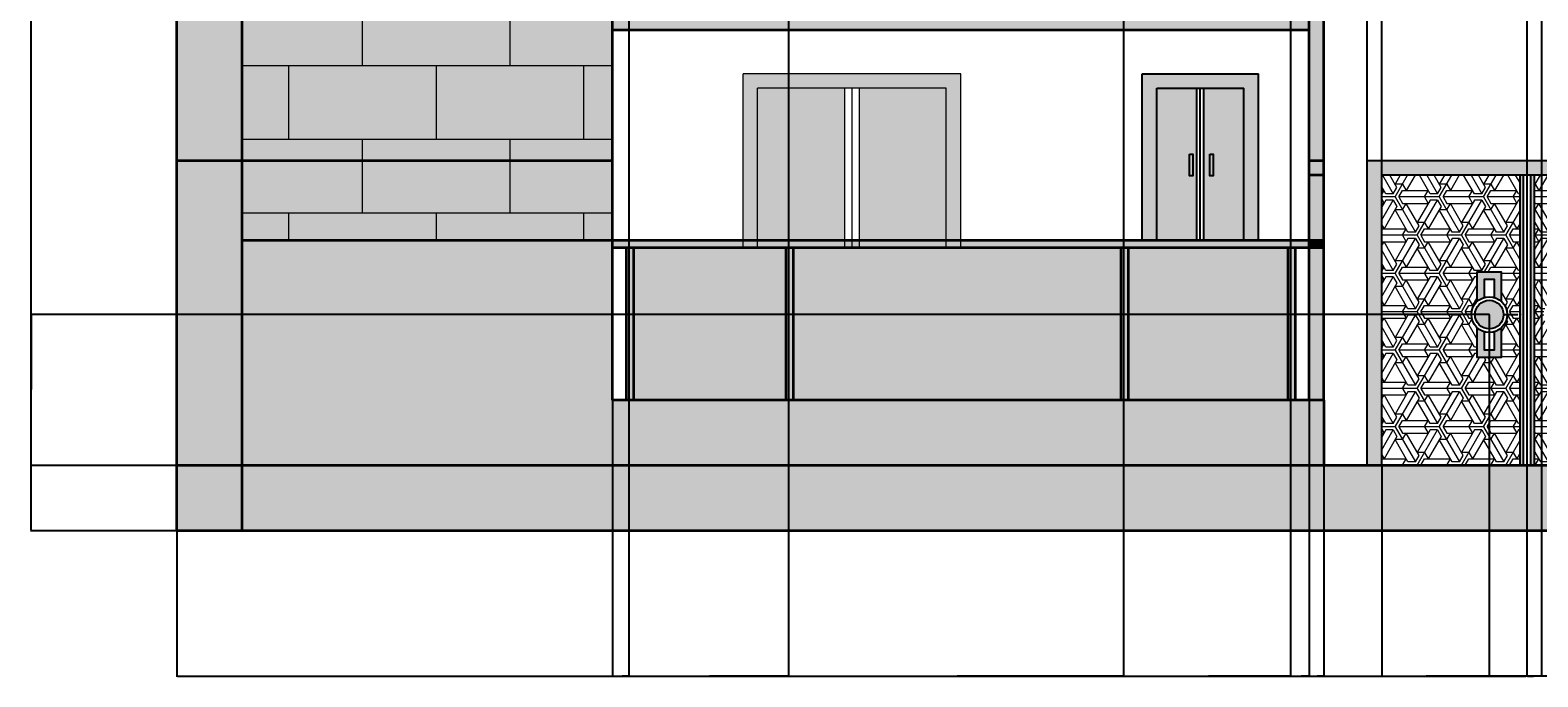
# Model space of a CAD drawing. Units: inches. Extents: x 2794 to 3619, y 522 to 1397.
# Tile 1 of 10: x 2794 to 3209, y 522 to 701. Entities that reach past the tile are written whole.
import ezdxf

# ---------------------------------------------------------------- set-up
doc = ezdxf.new("R2010")
doc.units = ezdxf.units.IN
for name, color, linetype, lineweight in [('A-ANNO-DIMS', 2, 'Continuous', 18), ('A-DOOR', 3, 'Continuous', 25), ('A-ELEV', 7, 'Continuous', 35), ('A-ELEV-PATT', 8, 'Continuous', 13), ('A-GLAZ', 4, 'Continuous', 18)]:
    doc.layers.add(name, color=color, linetype=linetype, lineweight=lineweight)
doc.styles.get("Standard").update_dxf_attribs({"font": 'arial.ttf'})
doc.dimstyles.get("Standard").update_dxf_attribs({"dimtxt": 0.18, "dimasz": 0.18, "dimexe": 0.18, "dimexo": 0.0625, "dimgap": 0.09, "dimtad": 0, "dimtih": 1, "dimtoh": 1, "dimdec": 4, "dimzin": 0, "dimdsep": 46, "dimtxsty": 'Standard', "dimcen": 0.09, "dimadec": 0, "dimazin": 0, "dimtfac": 1, "dimtdec": 4, "dimtofl": 0, "dimtmove": 0, "dimatfit": 3, "dimfxl": 1, "dimtolj": 1, "dimtzin": 0, "dimarcsym": 0})

# ---------------------------------------------------------------- blocks, each defined once
blk = doc.blocks.new('WIN-1500')
at = {"transparency": 33554646}
h = blk.add_hatch(color=256, dxfattribs=at)
h.dxf.hatch_style = 1
h.paths.add_polyline_path([(60, 48), (0, 48), (0, 2), (4, 2), (4, 44), (56, 44), (56, 2), (60, 2)])
at = {"transparency": 33554687}
h = blk.add_hatch(color=256, dxfattribs=at)
h.dxf.hatch_style = 1
h.set_gradient(color1=(248, 246, 176), color2=(74, 13, 14), name='INVCYLINDER')
h.paths.add_polyline_path([(56, 44), (32, 44), (32, 2), (56, 2)])
h.paths.add_polyline_path([(28, 44), (4, 44), (4, 2), (28, 2)])
for p, q in [((0, 0), (0, 48)), ((60, 48), (0, 48)), ((60, 0), (60, 48)), ((56, 44), (4, 44)), ((4, 0), (4, 44)), ((28, 44), (28, 0)), ((30, 44), (30, 0)), ((32, 44), (32, 0)), ((56, 0), (56, 44))]:
    blk.add_line(p, q)
blk = doc.blocks.new('DOOR-BALCONY-DBL')
at = {"transparency": 33554628}
h = blk.add_hatch(color=256, dxfattribs=at)
h.dxf.hatch_style = 1
h.paths.add_polyline_path([(4, 42), (28, 42), (28, 0), (32, 0), (32, 46), (0, 46), (0, 0), (4, 0)])
at = {"transparency": 33554646}
h = blk.add_hatch(color=256, dxfattribs=at)
h.dxf.hatch_style = 1
h.set_gradient(color1=(255, 255, 255), color2=(147, 149, 152), name='INVCYLINDER')
h.paths.add_polyline_path([(15, 42), (4, 42), (4, 0), (15, 0)])
h = blk.add_hatch(color=256, dxfattribs=at)
h.dxf.hatch_style = 1
h.set_gradient(color1=(255, 255, 255), color2=(147, 149, 152), name='INVCYLINDER')
h.paths.add_polyline_path([(28, 42), (17, 42), (17, 0), (28, 0)])
for p, q in [((0, 0), (0, 46)), ((0, 46), (32, 46)), ((4, 46), (28, 46)), ((32, 0), (32, 46)), ((4, 0), (4, 42)), ((4, 42), (28, 42)), ((15, 0), (15, 42)), ((16, 0), (16, 42)), ((17, 0), (17, 42)), ((28, 0), (28, 42))]:
    blk.add_line(p, q)
for points in [[(12.99, 23.83), (13.93, 23.83), (13.93, 17.87), (12.99, 17.87)], [(18.59, 23.83), (19.53, 23.83), (19.53, 17.87), (18.59, 17.87)]]:
    blk.add_lwpolyline(points, close=True)
blk = doc.blocks.new('*D7')
at = {"layer": 'A-ANNO-DIMS', "color": 0, "lineweight": -2, "transparency": 16777216}
for p, q in [((2834.27, 562.57), (2834.27, 522.36)), ((3578.27, 562.57), (3578.27, 522.36)), ((2834.45, 522.54), (3205.98, 522.54)), ((3578.09, 522.54), (3206.55, 522.54))]:
    blk.add_line(p, q, dxfattribs=at)
at = {"layer": 'A-ANNO-DIMS', "color": 0, "transparency": 16777216}
for points in [[(2834.45, 522.57), (2834.45, 522.51), (2834.27, 522.54)], [(3578.09, 522.57), (3578.09, 522.51), (3578.27, 522.54)]]:
    blk.add_solid(points, dxfattribs=at)
at = {"layer": 'Defpoints', "color": 0, "transparency": 16777216}
for p in [(2834.27, 562.64), (3578.27, 562.64), (3578.27, 522.54)]:
    blk.add_point(p, dxfattribs=at)
at = {"layer": 'A-ANNO-DIMS', "color": 0, "transparency": 16777216, "insert": (3206.27, 522.54), "char_height": 0.18, "attachment_point": 5}
blk.add_mtext('\\A1;744', dxfattribs=at)
blk = doc.blocks.new('*D16')
at = {"layer": 'A-ANNO-DIMS', "color": 0, "lineweight": -2, "transparency": 16777216}
for p, q in [((3142.2, 1356.64), (2793.99, 1356.64)), ((2794.17, 1356.46), (2794.17, 959.82)), ((2794.17, 562.82), (2794.17, 959.45)), ((2834.2, 562.64), (2793.99, 562.64))]:
    blk.add_line(p, q, dxfattribs=at)
at = {"layer": 'A-ANNO-DIMS', "color": 0, "transparency": 16777216}
for points in [[(2794.14, 1356.46), (2794.2, 1356.46), (2794.17, 1356.64)], [(2794.14, 562.82), (2794.2, 562.82), (2794.17, 562.64)]]:
    blk.add_solid(points, dxfattribs=at)
at = {"layer": 'Defpoints', "color": 0, "transparency": 16777216}
for p in [(2794.17, 1356.64), (3142.27, 1356.64), (2834.27, 562.64)]:
    blk.add_point(p, dxfattribs=at)
at = {"layer": 'A-ANNO-DIMS', "color": 0, "transparency": 16777216, "insert": (2794.17, 959.64), "char_height": 0.18, "attachment_point": 5}
blk.add_mtext('\\A1;794', dxfattribs=at)
blk = doc.blocks.new('*D32')
at = {"layer": 'A-ANNO-DIMS', "color": 0, "lineweight": -2, "transparency": 16777216}
for p, q in [((2954.27, 772.57), (2954.27, 522.36)), ((2958.83, 730.57), (2958.83, 522.36)), ((2954.45, 522.54), (2956.17, 522.54)), ((2958.65, 522.54), (2956.93, 522.54))]:
    blk.add_line(p, q, dxfattribs=at)
at = {"layer": 'A-ANNO-DIMS', "color": 0, "transparency": 16777216}
for points in [[(2954.45, 522.57), (2954.45, 522.51), (2954.27, 522.54)], [(2958.65, 522.57), (2958.65, 522.51), (2958.83, 522.54)]]:
    blk.add_solid(points, dxfattribs=at)
at = {"layer": 'Defpoints', "color": 0, "transparency": 16777216}
for p in [(2954.27, 772.64), (2958.83, 730.64), (2958.83, 522.54)]:
    blk.add_point(p, dxfattribs=at)
at = {"layer": 'A-ANNO-DIMS', "color": 0, "transparency": 16777216, "insert": (2956.55, 522.54), "char_height": 0.18, "attachment_point": 5}
blk.add_mtext('\\A1;4.561', dxfattribs=at)
blk = doc.blocks.new('*D33')
at = {"layer": 'A-ANNO-DIMS', "color": 0, "lineweight": -2, "transparency": 16777216}
for p, q in [((2958.83, 730.57), (2958.83, 522.36)), ((3002.83, 730.57), (3002.83, 522.36)), ((2959.01, 522.54), (2980.6, 522.54)), ((3002.65, 522.54), (2981.05, 522.54))]:
    blk.add_line(p, q, dxfattribs=at)
at = {"layer": 'A-ANNO-DIMS', "color": 0, "transparency": 16777216}
for points in [[(2959.01, 522.57), (2959.01, 522.51), (2958.83, 522.54)], [(3002.65, 522.57), (3002.65, 522.51), (3002.83, 522.54)]]:
    blk.add_solid(points, dxfattribs=at)
at = {"layer": 'Defpoints', "color": 0, "transparency": 16777216}
for p in [(2958.83, 730.64), (3002.83, 730.64), (3002.83, 522.54)]:
    blk.add_point(p, dxfattribs=at)
at = {"layer": 'A-ANNO-DIMS', "color": 0, "transparency": 16777216, "insert": (2980.83, 522.54), "char_height": 0.18, "attachment_point": 5}
blk.add_mtext('\\A1;44', dxfattribs=at)
blk = doc.blocks.new('*D34')
at = {"layer": 'A-ANNO-DIMS', "color": 0, "lineweight": -2, "transparency": 16777216}
for p, q in [((3002.83, 730.57), (3002.83, 522.36)), ((3095.13, 730.57), (3095.13, 522.36)), ((3003.01, 522.54), (3048.66, 522.54)), ((3094.95, 522.54), (3049.3, 522.54))]:
    blk.add_line(p, q, dxfattribs=at)
at = {"layer": 'A-ANNO-DIMS', "color": 0, "transparency": 16777216}
for points in [[(3003.01, 522.57), (3003.01, 522.51), (3002.83, 522.54)], [(3094.95, 522.57), (3094.95, 522.51), (3095.13, 522.54)]]:
    blk.add_solid(points, dxfattribs=at)
at = {"layer": 'Defpoints', "color": 0, "transparency": 16777216}
for p in [(3002.83, 730.64), (3095.13, 730.64), (3095.13, 522.54)]:
    blk.add_point(p, dxfattribs=at)
at = {"layer": 'A-ANNO-DIMS', "color": 0, "transparency": 16777216, "insert": (3048.98, 522.54), "char_height": 0.18, "attachment_point": 5}
blk.add_mtext('\\A1;92.3', dxfattribs=at)
blk = doc.blocks.new('*D35')
at = {"layer": 'A-ANNO-DIMS', "color": 0, "lineweight": -2, "transparency": 16777216}
for p, q in [((3095.13, 730.57), (3095.13, 522.36)), ((3141.11, 730.57), (3141.11, 522.36)), ((3095.31, 522.54), (3117.72, 522.54)), ((3140.93, 522.54), (3118.52, 522.54))]:
    blk.add_line(p, q, dxfattribs=at)
at = {"layer": 'A-ANNO-DIMS', "color": 0, "transparency": 16777216}
for points in [[(3095.31, 522.57), (3095.31, 522.51), (3095.13, 522.54)], [(3140.93, 522.57), (3140.93, 522.51), (3141.11, 522.54)]]:
    blk.add_solid(points, dxfattribs=at)
at = {"layer": 'Defpoints', "color": 0, "transparency": 16777216}
for p in [(3095.13, 730.64), (3141.11, 730.64), (3141.11, 522.54)]:
    blk.add_point(p, dxfattribs=at)
at = {"layer": 'A-ANNO-DIMS', "color": 0, "transparency": 16777216, "insert": (3118.12, 522.54), "char_height": 0.18, "attachment_point": 5}
blk.add_mtext('\\A1;45.98', dxfattribs=at)
blk = doc.blocks.new('*D36')
at = {"layer": 'A-ANNO-DIMS', "color": 0, "lineweight": -2, "transparency": 16777216}
for p, q in [((3146.27, 772.57), (3146.27, 522.36)), ((3141.11, 730.57), (3141.11, 522.36)), ((3141.29, 522.54), (3143.3, 522.54)), ((3146.09, 522.54), (3144.08, 522.54))]:
    blk.add_line(p, q, dxfattribs=at)
at = {"layer": 'A-ANNO-DIMS', "color": 0, "transparency": 16777216}
for points in [[(3141.29, 522.57), (3141.29, 522.51), (3141.11, 522.54)], [(3146.09, 522.57), (3146.09, 522.51), (3146.27, 522.54)]]:
    blk.add_solid(points, dxfattribs=at)
at = {"layer": 'Defpoints', "color": 0, "transparency": 16777216}
for p in [(3146.27, 772.64), (3141.11, 730.64), (3146.27, 522.54)]:
    blk.add_point(p, dxfattribs=at)
at = {"layer": 'A-ANNO-DIMS', "color": 0, "transparency": 16777216, "insert": (3143.69, 522.54), "char_height": 0.18, "attachment_point": 5}
blk.add_mtext('\\A1;5.154', dxfattribs=at)
blk = doc.blocks.new('*D49')
at = {"layer": 'A-ANNO-DIMS', "color": 0, "lineweight": -2, "transparency": 16777216}
for p, q in [((3146.27, 1256.19), (3146.27, 522.36)), ((3150.27, 1254.57), (3150.27, 522.36)), ((3146.45, 522.54), (3148.11, 522.54)), ((3150.09, 522.54), (3148.42, 522.54))]:
    blk.add_line(p, q, dxfattribs=at)
at = {"layer": 'A-ANNO-DIMS', "color": 0, "transparency": 16777216}
for points in [[(3146.45, 522.57), (3146.45, 522.51), (3146.27, 522.54)], [(3150.09, 522.57), (3150.09, 522.51), (3150.27, 522.54)]]:
    blk.add_solid(points, dxfattribs=at)
at = {"layer": 'Defpoints', "color": 0, "transparency": 16777216}
for p in [(3146.27, 1256.25), (3150.27, 1254.64), (3150.27, 522.54)]:
    blk.add_point(p, dxfattribs=at)
at = {"layer": 'A-ANNO-DIMS', "color": 0, "transparency": 16777216, "insert": (3148.27, 522.54), "char_height": 0.18, "attachment_point": 5}
blk.add_mtext('\\A1;4', dxfattribs=at)
blk = doc.blocks.new('*D50')
at = {"layer": 'A-ANNO-DIMS', "color": 0, "lineweight": -2, "transparency": 16777216}
for p, q in [((3150.27, 1254.57), (3150.27, 522.36)), ((3206.27, 1254.57), (3206.27, 522.36)), ((3150.45, 522.54), (3178.05, 522.54)), ((3206.09, 522.54), (3178.48, 522.54))]:
    blk.add_line(p, q, dxfattribs=at)
at = {"layer": 'A-ANNO-DIMS', "color": 0, "transparency": 16777216}
for points in [[(3150.45, 522.57), (3150.45, 522.51), (3150.27, 522.54)], [(3206.09, 522.57), (3206.09, 522.51), (3206.27, 522.54)]]:
    blk.add_solid(points, dxfattribs=at)
at = {"layer": 'Defpoints', "color": 0, "transparency": 16777216}
for p in [(3150.27, 1254.64), (3206.27, 1254.64), (3206.27, 522.54)]:
    blk.add_point(p, dxfattribs=at)
at = {"layer": 'A-ANNO-DIMS', "color": 0, "transparency": 16777216, "insert": (3178.27, 522.54), "char_height": 0.18, "attachment_point": 5}
blk.add_mtext('\\A1;56', dxfattribs=at)
blk = doc.blocks.new('*D51')
at = {"layer": 'A-ANNO-DIMS', "color": 0, "lineweight": -2, "transparency": 16777216}
for p, q in [((3206.27, 1254.57), (3206.27, 522.36)), ((3210.27, 1254.57), (3210.27, 522.36)), ((3206.45, 522.54), (3208.11, 522.54)), ((3210.09, 522.54), (3208.42, 522.54))]:
    blk.add_line(p, q, dxfattribs=at)
at = {"layer": 'A-ANNO-DIMS', "color": 0, "transparency": 16777216}
for points in [[(3206.45, 522.57), (3206.45, 522.51), (3206.27, 522.54)], [(3210.09, 522.57), (3210.09, 522.51), (3210.27, 522.54)]]:
    blk.add_solid(points, dxfattribs=at)
at = {"layer": 'Defpoints', "color": 0, "transparency": 16777216}
for p in [(3206.27, 1254.64), (3210.27, 1254.64), (3210.27, 522.54)]:
    blk.add_point(p, dxfattribs=at)
at = {"layer": 'A-ANNO-DIMS', "color": 0, "transparency": 16777216, "insert": (3208.27, 522.54), "char_height": 0.18, "attachment_point": 5}
blk.add_mtext('\\A1;4', dxfattribs=at)
blk = doc.blocks.new('*D56')
at = {"layer": 'A-ANNO-DIMS', "color": 0, "lineweight": -2, "transparency": 16777216}
for p, q in [((3162.27, 664.7), (3162.27, 1396.92)), ((3162.45, 1396.74), (3206.05, 1396.74)), ((3250.09, 1396.74), (3206.49, 1396.74)), ((3250.27, 664.7), (3250.27, 1396.92))]:
    blk.add_line(p, q, dxfattribs=at)
at = {"layer": 'A-ANNO-DIMS', "color": 0, "transparency": 16777216}
for points in [[(3162.45, 1396.77), (3162.45, 1396.71), (3162.27, 1396.74)], [(3250.09, 1396.77), (3250.09, 1396.71), (3250.27, 1396.74)]]:
    blk.add_solid(points, dxfattribs=at)
at = {"layer": 'Defpoints', "color": 0, "transparency": 16777216}
for p in [(3250.27, 1396.74), (3162.27, 664.64), (3250.27, 664.64)]:
    blk.add_point(p, dxfattribs=at)
at = {"layer": 'A-ANNO-DIMS', "color": 0, "transparency": 16777216, "insert": (3206.27, 1396.74), "char_height": 0.18, "attachment_point": 5}
blk.add_mtext('\\A1;88', dxfattribs=at)
blk = doc.blocks.new('*D57')
at = {"layer": 'A-ANNO-DIMS', "color": 0, "lineweight": -2, "transparency": 16777216}
for p, q in [((3162.27, 664.7), (3162.27, 1396.92)), ((3162.45, 1396.74), (3164.11, 1396.74)), ((3166.09, 1396.74), (3164.42, 1396.74)), ((3166.27, 660.7), (3166.27, 1396.92))]:
    blk.add_line(p, q, dxfattribs=at)
at = {"layer": 'A-ANNO-DIMS', "color": 0, "transparency": 16777216}
for points in [[(3162.45, 1396.77), (3162.45, 1396.71), (3162.27, 1396.74)], [(3166.09, 1396.77), (3166.09, 1396.71), (3166.27, 1396.74)]]:
    blk.add_solid(points, dxfattribs=at)
at = {"layer": 'Defpoints', "color": 0, "transparency": 16777216}
for p in [(3166.27, 1396.74), (3162.27, 664.64), (3166.27, 660.64)]:
    blk.add_point(p, dxfattribs=at)
at = {"layer": 'A-ANNO-DIMS', "color": 0, "transparency": 16777216, "insert": (3164.27, 1396.74), "char_height": 0.18, "attachment_point": 5}
blk.add_mtext('\\A1;4', dxfattribs=at)
blk = doc.blocks.new('*D58')
at = {"layer": 'A-ANNO-DIMS', "color": 0, "lineweight": -2, "transparency": 16777216}
for p, q in [((3150.27, 580.7), (3150.27, 1396.92)), ((3150.45, 1396.74), (3156.06, 1396.74)), ((3162.09, 1396.74), (3156.48, 1396.74)), ((3162.27, 664.7), (3162.27, 1396.92))]:
    blk.add_line(p, q, dxfattribs=at)
at = {"layer": 'A-ANNO-DIMS', "color": 0, "transparency": 16777216}
for points in [[(3150.45, 1396.77), (3150.45, 1396.71), (3150.27, 1396.74)], [(3162.09, 1396.77), (3162.09, 1396.71), (3162.27, 1396.74)]]:
    blk.add_solid(points, dxfattribs=at)
at = {"layer": 'Defpoints', "color": 0, "transparency": 16777216}
for p in [(3162.27, 1396.74), (3162.27, 664.64), (3150.27, 580.64)]:
    blk.add_point(p, dxfattribs=at)
at = {"layer": 'A-ANNO-DIMS', "color": 0, "transparency": 16777216, "insert": (3156.27, 1396.74), "char_height": 0.18, "attachment_point": 5}
blk.add_mtext('\\A1;12', dxfattribs=at)
blk = doc.blocks.new('*D61')
at = {"layer": 'A-ANNO-DIMS', "color": 0, "lineweight": -2, "transparency": 16777216}
for p, q in [((3195.89, 622.15), (3195.89, 522.36)), ((3166.27, 580.57), (3166.27, 522.36)), ((3166.45, 522.54), (3180.61, 522.54)), ((3195.71, 522.54), (3181.54, 522.54))]:
    blk.add_line(p, q, dxfattribs=at)
at = {"layer": 'A-ANNO-DIMS', "color": 0, "transparency": 16777216}
for points in [[(3166.45, 522.57), (3166.45, 522.51), (3166.27, 522.54)], [(3195.71, 522.57), (3195.71, 522.51), (3195.89, 522.54)]]:
    blk.add_solid(points, dxfattribs=at)
at = {"layer": 'Defpoints', "color": 0, "transparency": 16777216}
for p in [(3195.89, 622.22), (3166.27, 580.64), (3195.89, 522.54)]:
    blk.add_point(p, dxfattribs=at)
at = {"layer": 'A-ANNO-DIMS', "color": 0, "transparency": 16777216, "insert": (3181.08, 522.54), "char_height": 0.18, "attachment_point": 5}
blk.add_mtext('\\A1;29.627', dxfattribs=at)
blk = doc.blocks.new('*D63')
at = {"layer": 'A-ANNO-DIMS', "color": 0, "lineweight": -2, "transparency": 16777216}
for p, q in [((3195.83, 622.22), (2793.99, 622.22)), ((2794.17, 622.04), (2794.17, 601.61)), ((2794.17, 580.82), (2794.17, 601.24)), ((3166.2, 580.64), (2793.99, 580.64))]:
    blk.add_line(p, q, dxfattribs=at)
at = {"layer": 'A-ANNO-DIMS', "color": 0, "transparency": 16777216}
for points in [[(2794.14, 622.04), (2794.2, 622.04), (2794.17, 622.22)], [(2794.14, 580.82), (2794.2, 580.82), (2794.17, 580.64)]]:
    blk.add_solid(points, dxfattribs=at)
at = {"layer": 'Defpoints', "color": 0, "transparency": 16777216}
for p in [(2794.17, 622.22), (3195.89, 622.22), (3166.27, 580.64)]:
    blk.add_point(p, dxfattribs=at)
at = {"layer": 'A-ANNO-DIMS', "color": 0, "transparency": 16777216, "insert": (2794.17, 601.43), "char_height": 0.18, "attachment_point": 5}
blk.add_mtext('\\A1;41.58', dxfattribs=at)
blk = doc.blocks.new('*D66')
at = {"layer": 'A-ANNO-DIMS', "color": 0, "lineweight": -2, "transparency": 16777216}
for p, q in [((3195.8, 622.22), (3195.98, 622.22)), ((3195.89, 622.13), (3195.89, 622.31)), ((3203.79, 622.19), (3201.01, 622.2))]:
    blk.add_line(p, q, dxfattribs=at)
at = {"layer": 'A-ANNO-DIMS', "color": 0, "transparency": 16777216}
blk.add_solid([(3201.01, 622.23), (3201.01, 622.17), (3200.83, 622.2)], dxfattribs=at)
at = {"layer": 'Defpoints', "color": 0, "transparency": 16777216}
for p in [(3190.96, 622.23), (3200.83, 622.2)]:
    blk.add_point(p, dxfattribs=at)
at = {"layer": 'A-ANNO-DIMS', "color": 0, "transparency": 16777216, "insert": (3204.47, 622.19), "char_height": 0.18, "attachment_point": 5}
blk.add_mtext('\\A1;2X ∅9.872', dxfattribs=at)
blk = doc.blocks.new('*D67')
at = {"layer": 'A-ANNO-DIMS', "color": 0, "lineweight": -2, "transparency": 16777216}
for p, q in [((3195.8, 622.22), (3195.98, 622.22)), ((3195.89, 622.13), (3195.89, 622.31)), ((3202.19, 622.19), (3200.01, 622.2))]:
    blk.add_line(p, q, dxfattribs=at)
at = {"layer": 'A-ANNO-DIMS', "color": 0, "transparency": 16777216}
blk.add_solid([(3200.01, 622.23), (3200.01, 622.17), (3199.83, 622.2)], dxfattribs=at)
at = {"layer": 'Defpoints', "color": 0, "transparency": 16777216}
for p in [(3191.96, 622.23), (3199.83, 622.2)]:
    blk.add_point(p, dxfattribs=at)
at = {"layer": 'A-ANNO-DIMS', "color": 0, "transparency": 16777216, "insert": (3202.87, 622.19), "char_height": 0.18, "attachment_point": 5}
blk.add_mtext('\\A1;2X ∅7.872', dxfattribs=at)

msp = doc.modelspace()

# ---------------------------------------------------------------- hatches: boundary and pattern name
at = {"layer": 'A-ELEV-PATT', "transparency": 33554687}
h = msp.add_hatch(color=256, dxfattribs=at)
h.dxf.hatch_style = 1
h.paths.add_polyline_path([(3578.2659, 1294.6351), (3560.2659, 1294.6351), (3560.2659, 642.6351), (3578.2659, 642.6351)])
h.paths.add_polyline_path([(2852.2659, 1294.6351), (2834.2659, 1294.6351), (2834.2659, 642.6351), (2852.2659, 642.6351)])
h = msp.add_hatch(color=256, dxfattribs=at)
h.dxf.hatch_style = 1
h.paths.add_polyline_path([(2852.2659, 1294.6351), (2834.2659, 1294.6351), (2834.2659, 562.6351), (2852.2659, 562.6351)])
h.paths.add_polyline_path([(3578.2659, 1294.6351), (3560.2659, 1294.6351), (3560.2659, 562.6351), (3578.2659, 562.6351)])
h = msp.add_hatch(color=256, dxfattribs=at)
h.dxf.hatch_style = 1
h.paths.add_polyline_path([(3146.2659, 1096.6351), (3146.2659, 1126.6351), (2954.2659, 1126.6351), (2954.2659, 1096.6351)])
h.paths.add_polyline_path([(3458.2659, 1096.6351), (3458.2659, 1126.6351), (3266.2659, 1126.6351), (3266.2659, 1096.6351)])
h.paths.add_polyline_path([(3458.2659, 964.6351), (3458.2659, 994.6351), (3266.2659, 994.6351), (3266.2659, 964.6351)])
h.paths.add_polyline_path([(3146.2659, 964.6351), (3146.2659, 994.6351), (2954.2659, 994.6351), (2954.2659, 964.6351)])
h.paths.add_polyline_path([(3458.2659, 832.6351), (3458.2659, 862.6351), (3266.2659, 862.6351), (3266.2659, 832.6351)])
h.paths.add_polyline_path([(3146.2659, 832.6351), (3146.2659, 862.6351), (2954.2659, 862.6351), (2954.2659, 832.6351)])
h.paths.add_polyline_path([(3458.2659, 700.6351), (3458.2659, 730.6351), (3266.2659, 730.6351), (3266.2659, 700.6351)])
h.paths.add_polyline_path([(3146.2659, 700.6351), (3146.2659, 730.6351), (2954.2659, 730.6351), (2954.2659, 700.6351)])
h.paths.add_polyline_path([(3266.2659, 1294.6351), (3266.2659, 1258.6351), (3266.2659, 1228.6351), (3458.2659, 1228.6351), (3458.2659, 1294.6351)])
h.paths.add_polyline_path([(3146.2659, 1228.6351), (3146.2659, 1256.2485, -0.00994307), (3146.2659, 1258.6351), (3146.2659, 1294.6351), (2954.2659, 1294.6351), (2954.2659, 1228.6351)])
at = {"layer": 'A-ELEV-PATT'}
h = msp.add_hatch(dxfattribs=at)
h.set_pattern_fill('AR-B816', color=256, scale=0.1)
h.paths.add_polyline_path([(2954.2659, 1114.6351), (2852.2659, 1114.6351), (2852.2659, 994.6351), (2954.2659, 994.6351)])
h.paths.add_polyline_path([(2954.2659, 1246.6351), (2852.2659, 1246.6351), (2852.2659, 1126.6351), (2954.2659, 1126.6351)])
h.paths.add_polyline_path([(2954.2659, 982.6351), (2852.2659, 982.6351), (2852.2659, 862.6351), (2954.2659, 862.6351)])
h.paths.add_polyline_path([(2954.2659, 850.6351), (2852.2659, 850.6351), (2852.2659, 730.6351), (2954.2659, 730.6351)])
h.paths.add_polyline_path([(3560.2659, 850.6351), (3458.2659, 850.6351), (3458.2659, 730.6351), (3560.2659, 730.6351)])
h.paths.add_polyline_path([(3560.2659, 982.6351), (3458.2659, 982.6351), (3458.2659, 862.6351), (3560.2659, 862.6351)])
h.paths.add_polyline_path([(3560.2659, 1114.6351), (3458.2659, 1114.6351), (3458.2659, 994.6351), (3560.2659, 994.6351)])
h.paths.add_polyline_path([(3560.2659, 1246.6351), (3458.2659, 1246.6351), (3458.2659, 1126.6351), (3560.2659, 1126.6351)])
h.paths.add_polyline_path([(2852.2659, 642.6351), (2954.2659, 642.6351), (2954.2659, 718.6351), (2852.2659, 718.6351)])
h.paths.add_polyline_path([(3458.2659, 640.6351), (3560.2659, 640.6351), (3560.2659, 718.6351), (3458.2659, 718.6351)])
at = {"layer": 'A-ELEV-PATT', "transparency": 33554630}
h = msp.add_hatch(color=256, dxfattribs=at)
h.dxf.hatch_style = 1
h.paths.add_polyline_path([(2954.2659, 1114.6351), (2852.2659, 1114.6351), (2852.2659, 994.6351), (2954.2659, 994.6351)])
h.paths.add_polyline_path([(2954.2659, 982.6351), (2852.2659, 982.6351), (2852.2659, 862.6351), (2954.2659, 862.6351)])
h.paths.add_polyline_path([(2954.2659, 850.6351), (2852.2659, 850.6351), (2852.2659, 730.6351), (2954.2659, 730.6351)])
h.paths.add_polyline_path([(3560.2659, 850.6351), (3458.2659, 850.6351), (3458.2659, 730.6351), (3560.2659, 730.6351)])
h.paths.add_polyline_path([(3560.2659, 982.6351), (3458.2659, 982.6351), (3458.2659, 862.6351), (3560.2659, 862.6351)])
h.paths.add_polyline_path([(3560.2659, 1114.6351), (3458.2659, 1114.6351), (3458.2659, 994.6351), (3560.2659, 994.6351)])
h.paths.add_polyline_path([(3560.2659, 1246.6351), (3458.2659, 1246.6351), (3458.2659, 1126.6351), (3560.2659, 1126.6351)])
h.paths.add_polyline_path([(2852.2659, 642.6351), (2954.2659, 642.6351), (2954.2659, 718.6351), (2852.2659, 718.6351)])
h.paths.add_polyline_path([(3458.2659, 642.6351), (3560.2659, 642.6351), (3560.2659, 718.6351), (3458.2659, 718.6351)])
at = {"layer": 'A-ELEV-PATT', "transparency": 33554687}
h = msp.add_hatch(color=256, dxfattribs=at)
h.dxf.hatch_style = 1
h.paths.add_polyline_path([(3150.2659, 730.6351), (3146.2659, 730.6351), (3146.2659, 642.6351), (3150.2659, 642.6351)])
h = msp.add_hatch(color=256, dxfattribs=at)
h.dxf.hatch_style = 1
h.paths.add_polyline_path([(3266.2659, 700.6351), (3262.2659, 700.6351), (3262.2659, 642.6351), (3266.2659, 642.6351)])
h.paths.add_polyline_path([(3266.2659, 640.6351), (3262.2659, 640.6351), (3262.2659, 598.6351), (3266.2659, 598.6351)])
h.paths.add_polyline_path([(3458.2659, 642.6351), (3266.2659, 642.6351), (3266.2659, 640.6351), (3458.2659, 640.6351)])
h.paths.add_polyline_path([(3272.4761, 640.6351), (3270.4761, 640.6351), (3270.4761, 598.6351), (3272.4761, 598.6351)])
h.paths.add_polyline_path([(3316.4761, 640.6351), (3314.4761, 640.6351), (3314.4761, 598.6351), (3316.4761, 598.6351)])
h.paths.add_polyline_path([(3266.2659, 642.6351), (3262.2659, 642.6351), (3262.2659, 640.6351), (3266.2659, 640.6351)])
h.paths.add_polyline_path([(3150.2659, 640.6351), (3146.2659, 640.6351), (3146.2659, 598.6351), (3150.2659, 598.6351)])
h = msp.add_hatch(color=256, dxfattribs=at)
h.dxf.hatch_style = 1
h.paths.add_polyline_path([(3246.2659, 664.6351), (3166.2659, 664.6351), (3166.2659, 660.6351), (3246.2659, 660.6351)])
h.paths.add_polyline_path([(3166.2659, 660.6351), (3162.2659, 660.6351), (3162.2659, 580.6351), (3166.2659, 580.6351)])
h.paths.add_polyline_path([(3250.2659, 660.6351), (3246.2659, 660.6351), (3246.2659, 580.6351), (3250.2659, 580.6351)])
h = msp.add_hatch(color=256, dxfattribs=at)
h.dxf.hatch_style = 1
h.paths.add_polyline_path([(3166.2659, 664.6351), (3162.2659, 664.6351), (3162.2659, 660.6351), (3166.2659, 660.6351)])
h.paths.add_polyline_path([(3250.2659, 664.6351), (3246.2659, 664.6351), (3246.2659, 660.6351), (3250.2659, 660.6351)])
h = msp.add_hatch(dxfattribs=at)
h.set_pattern_fill('ESCHER', color=256, scale=0.4)
h.paths.add_polyline_path([(3204.2659, 660.6351), (3166.2659, 660.6351), (3166.2659, 580.6351), (3204.2659, 580.6351)])
h.paths.add_polyline_path([(3192.5875, 634.0076), (3199.1979, 634.0076), (3199.1979, 625.8832, -0.21239083), (3200.8288, 622.217, -0.21239083), (3199.1979, 618.5509), (3199.1979, 610.4265), (3192.5875, 610.4265), (3192.5875, 618.5509, -0.21239083), (3190.9566, 622.217, -0.21239083), (3192.5875, 625.8832)], flags=16)
h.paths.add_polyline_path([(3199.8288, 622.217, -1), (3191.9566, 622.217, -1)], flags=0)
h.paths.add_polyline_path([(3246.2659, 660.6351), (3208.2659, 660.6351), (3208.2659, 580.6351), (3246.2659, 580.6351)])
h.paths.add_polyline_path([(3219.1237, 634.0076), (3219.1237, 625.8832, -0.21239083), (3220.7546, 622.217, -0.21239083), (3219.1237, 618.5509), (3219.1237, 610.4265), (3212.5133, 610.4265), (3212.5133, 618.5509, -0.21239083), (3210.8824, 622.217, -0.21239083), (3212.5133, 625.8832), (3212.5133, 634.0076)], flags=16)
h.paths.add_polyline_path([(3219.7546, 622.217, -1), (3211.8824, 622.217, -1)], flags=0)
h = msp.add_hatch(color=256, dxfattribs=at)
h.dxf.hatch_style = 1
h.paths.add_polyline_path([(3208.2659, 660.6351), (3207.2659, 660.6351), (3207.2659, 580.6351), (3208.2659, 580.6351)])
h.paths.add_polyline_path([(3205.2659, 660.6351), (3204.2659, 660.6351), (3204.2659, 580.6351), (3205.2659, 580.6351)])
h = msp.add_hatch(color=256, dxfattribs=at)
h.dxf.hatch_style = 1
h.paths.add_polyline_path([(2954.2659, 642.6351), (2852.2659, 642.6351), (2852.2659, 598.6351), (2954.2659, 598.6351)])
h.paths.add_polyline_path([(3150.2659, 598.6351), (2852.2659, 598.6351), (2852.2659, 580.6351), (3150.2659, 580.6351)])
h.paths.add_polyline_path([(3560.2659, 642.6351), (3458.2659, 642.6351), (3458.2659, 598.6351), (3560.2659, 598.6351)])
h.paths.add_polyline_path([(3560.2659, 598.6351), (3262.2659, 598.6351), (3262.2659, 580.6351), (3560.2659, 580.6351)])
h = msp.add_hatch(color=256, dxfattribs=at)
h.dxf.hatch_style = 1
h.paths.add_polyline_path([(3142.3604, 640.6351), (3140.3604, 640.6351), (3140.3604, 598.6351), (3142.3604, 598.6351)])
h.paths.add_polyline_path([(3146.2659, 642.6351), (2954.2659, 642.6351), (2954.2659, 640.6351), (3146.2659, 640.6351)])
h.paths.add_polyline_path([(3096.3813, 640.6351), (3094.3813, 640.6351), (3094.3813, 598.6351), (3096.3813, 598.6351)])
h.paths.add_polyline_path([(3004.0752, 640.6351), (3002.0752, 640.6351), (3002.0752, 598.6351), (3004.0752, 598.6351)])
h.paths.add_polyline_path([(2960.0752, 640.6351), (2958.0752, 640.6351), (2958.0752, 598.6351), (2960.0752, 598.6351)])
h.paths.add_polyline_path([(3408.7822, 640.6351), (3406.7822, 640.6351), (3406.7822, 598.6351), (3408.7822, 598.6351)])
h.paths.add_polyline_path([(3454.7613, 640.6351), (3452.7613, 640.6351), (3452.7613, 598.6351), (3454.7613, 598.6351)])
h = msp.add_hatch(dxfattribs=at)
h.set_pattern_fill('EARTH', color=256)
h.paths.add_polyline_path([(3002.0752, 640.6351), (2960.0752, 640.6351), (2960.0752, 598.6351), (3002.0752, 598.6351)])
h.paths.add_polyline_path([(3094.3813, 640.6351), (3004.0752, 640.6351), (3004.0752, 598.6351), (3094.3813, 598.6351)])
h.paths.add_polyline_path([(3140.3604, 640.6351), (3096.3813, 640.6351), (3096.3813, 598.6351), (3140.3604, 598.6351)])
h.paths.add_polyline_path([(3314.4761, 640.6351), (3272.4761, 640.6351), (3272.4761, 598.6351), (3314.4761, 598.6351)])
h.paths.add_polyline_path([(3406.7822, 640.6351), (3316.4761, 640.6351), (3316.4761, 598.6351), (3406.7822, 598.6351)])
h.paths.add_polyline_path([(3452.7613, 640.6351), (3408.7822, 640.6351), (3408.7822, 598.6351), (3452.7613, 598.6351)])
h = msp.add_hatch(color=256, dxfattribs=at)
h.dxf.hatch_style = 1
h.paths.add_polyline_path([(3150.2659, 642.6351), (3146.2659, 642.6351), (3146.2659, 640.6351), (3150.2659, 640.6351)])
h = msp.add_hatch(color=256, dxfattribs=at)
h.dxf.hatch_style = 1
h.paths.add_polyline_path([(3199.1979, 634.0076), (3192.5875, 634.0076), (3192.5875, 625.8832, -0.11704667), (3194.5875, 626.9774), (3194.5875, 632.0076), (3197.1979, 632.0076), (3197.1979, 626.9774, -0.11704667), (3199.1979, 625.8832)])
h.paths.add_polyline_path([(3199.1979, 618.5509, -0.11704667), (3197.1979, 617.4566), (3197.1979, 612.4265), (3194.5875, 612.4265), (3194.5875, 617.4566, -0.11704667), (3192.5875, 618.5509), (3192.5875, 610.4265), (3199.1979, 610.4265)])
h.paths.add_polyline_path([(3191.9566, 622.217, 1), (3199.8288, 622.217, 1)])
h.paths.add_polyline_path([(3219.1237, 634.0076), (3212.5133, 634.0076), (3212.5133, 625.8832, -0.11704667), (3214.5133, 626.9774), (3214.5133, 632.0076), (3217.1237, 632.0076), (3217.1237, 626.9774, -0.11704667), (3219.1237, 625.8832)])
h.paths.add_polyline_path([(3219.1237, 618.5509, -0.11704667), (3217.1237, 617.4566), (3217.1237, 612.4265), (3214.5133, 612.4265), (3214.5133, 617.4566, -0.11704667), (3212.5133, 618.5509), (3212.5133, 610.4265), (3219.1237, 610.4265)])
h.paths.add_polyline_path([(3211.8824, 622.217, 1), (3219.7546, 622.217, 1)])
h = msp.add_hatch(color=256, dxfattribs=at)
h.dxf.hatch_style = 1
h.paths.add_polyline_path([(3560.2659, 580.6351), (2852.2659, 580.6351), (2852.2659, 562.6351), (3560.2659, 562.6351)])

# ---------------------------------------------------------------- linework, layer by layer
at = {"layer": 'A-DOOR'}
for p, q in [((3162.2659, 580.6351), (3162.2659, 664.6351)), ((3250.2659, 664.6351), (3162.2659, 664.6351)), ((3166.2659, 580.6351), (3166.2659, 660.6351)), ((3246.2659, 660.6351), (3166.2659, 660.6351)), ((3204.2659, 660.6351), (3204.2659, 580.6351)), ((3205.2659, 660.6351), (3205.2659, 580.6351)), ((3207.2659, 660.6351), (3207.2659, 580.6351)), ((3208.2659, 660.6351), (3208.2659, 580.6351))]:
    msp.add_line(p, q, dxfattribs=at)
for points in [[(3192.5875, 625.8832), (3192.5875, 634.0076), (3199.1979, 634.0076), (3199.1979, 625.8832)], [(3194.5875, 626.9774), (3194.5875, 632.0076), (3197.1979, 632.0076), (3197.1979, 626.9774)], [(3199.1979, 618.5509), (3199.1979, 610.4265), (3192.5875, 610.4265), (3192.5875, 618.5509)], [(3197.1979, 617.4566), (3197.1979, 612.4265), (3194.5875, 612.4265), (3194.5875, 617.4566)]]:
    msp.add_lwpolyline(points, dxfattribs=at)
for radius in [4.9361, 3.9361]:
    msp.add_circle((3195.8927, 622.217), radius, dxfattribs=at)
at = {"layer": 'A-ELEV'}
for p, q in [((2834.2659, 562.6351), (2834.2659, 1297.6351)), ((2852.2659, 562.6351), (2852.2659, 1294.6351)), ((2954.2659, 598.6351), (2954.2659, 1294.6351)), ((3146.2659, 598.6351), (3146.2659, 1258.6351)), ((3150.2659, 598.6351), (3150.2659, 1258.6351)), ((3146.2659, 700.6351), (2954.2659, 700.6351)), ((2954.2659, 664.6351), (2834.2659, 664.6351)), ((3150.2659, 664.6351), (3146.2659, 664.6351)), ((3150.2659, 660.6351), (3146.2659, 660.6351)), ((3150.2659, 642.6351), (2852.2659, 642.6351)), ((3150.2659, 640.6351), (2954.2659, 640.6351)), ((2958.0752, 640.6351), (2958.0752, 598.6351)), ((2960.0752, 640.6351), (2960.0752, 598.6351)), ((3002.0752, 640.6351), (3002.0752, 598.6351)), ((3004.0752, 640.6351), (3004.0752, 598.6351)), ((3094.3813, 640.6351), (3094.3813, 598.6351)), ((3096.3813, 640.6351), (3096.3813, 598.6351)), ((3140.3604, 640.6351), (3140.3604, 598.6351)), ((3142.3604, 640.6351), (3142.3604, 598.6351)), ((3150.2659, 598.6351), (2954.2659, 598.6351)), ((3150.2659, 598.6351), (3150.2659, 580.6351)), ((3578.2659, 580.6351), (2834.2659, 580.6351)), ((3578.2659, 562.6351), (2834.2659, 562.6351))]:
    msp.add_line(p, q, dxfattribs=at)

# ---------------------------------------------------------------- block references
at = {"layer": 'A-DOOR'}
msp.add_blockref('DOOR-BALCONY-DBL', (3100.266, 642.635), dxfattribs=at)
at = {"layer": 'A-GLAZ'}
msp.add_blockref('WIN-1500', (2990.266, 640.635), dxfattribs=at)

# ---------------------------------------------------------------- dimensions: what is measured, and where the dimension line sits
at = {"layer": 'A-ANNO-DIMS'}
for base, p1, p2, override, picture, middle in [((3162.2659, 1396.7351), (3150.2659, 580.6351), (3162.2659, 664.6351), {"dimdec": 0, "dimlfac": 1, "dimrnd": 0, "dimzin": 0, "dimdsep": 46, "dimlunit": 2}, '*D58', (3156.2659, 1396.7351)), ((3250.2659, 1396.7351), (3162.2659, 664.6351), (3250.2659, 664.6351), {"dimdec": 0, "dimlfac": 1, "dimrnd": 0, "dimzin": 0, "dimdsep": 46, "dimlunit": 2}, '*D56', (3206.2659, 1396.7351)), ((3166.2659, 1396.7351), (3162.2659, 664.6351), (3166.2659, 660.6351), {"dimdec": 0, "dimlfac": 1, "dimrnd": 0, "dimzin": 0, "dimdsep": 46, "dimlunit": 2}, '*D57', (3164.2659, 1396.7351)), ((3150.2659, 522.5351), (3146.2659, 1256.2485), (3150.2659, 1254.6351), {"dimdec": 0, "dimlfac": 1, "dimrnd": 0, "dimzin": 0, "dimdsep": 46, "dimlunit": 2}, '*D49', (3148.2659, 522.5351)), ((3206.2659, 522.5351), (3150.2659, 1254.6351), (3206.2659, 1254.6351), {"dimdec": 0, "dimlfac": 1, "dimrnd": 0, "dimzin": 0, "dimdsep": 46, "dimlunit": 2}, '*D50', (3178.2659, 522.5351)), ((3210.2659, 522.5351), (3206.2659, 1254.6351), (3210.2659, 1254.6351), {"dimdec": 0, "dimlfac": 1, "dimrnd": 0, "dimzin": 0, "dimdsep": 46, "dimlunit": 2}, '*D51', (3208.2659, 522.5351)), ((2958.8268, 522.5351), (2954.2659, 772.6351), (2958.8268, 730.6351), {"dimdec": 3, "dimlfac": 1, "dimrnd": 0, "dimzin": 0, "dimdsep": 46, "dimlunit": 2}, '*D32', (2956.5463, 522.5351)), ((3146.2659, 522.5351), (3141.112, 730.6351), (3146.2659, 772.6351), {"dimdec": 3, "dimlfac": 1, "dimrnd": 0, "dimzin": 0, "dimdsep": 46, "dimlunit": 2}, '*D36', (3143.6889, 522.5351)), ((3002.8268, 522.5351), (2958.8268, 730.6351), (3002.8268, 730.6351), {"dimdec": 0, "dimlfac": 1, "dimrnd": 0, "dimzin": 0, "dimdsep": 46, "dimlunit": 2}, '*D33', (2980.8268, 522.5351)), ((3095.1329, 522.5351), (3002.8268, 730.6351), (3095.1329, 730.6351), {"dimdec": 1, "dimlfac": 1, "dimrnd": 0, "dimzin": 0, "dimdsep": 46, "dimlunit": 2}, '*D34', (3048.9798, 522.5351)), ((3141.112, 522.5351), (3095.1329, 730.6351), (3141.112, 730.6351), {"dimdec": 2, "dimlfac": 1, "dimrnd": 0, "dimzin": 0, "dimdsep": 46, "dimlunit": 2}, '*D35', (3118.1224, 522.5351)), ((3195.8927, 522.5351), (3166.2659, 580.6351), (3195.8927, 622.217), {"dimdec": 3, "dimlfac": 1, "dimrnd": 0, "dimzin": 0, "dimdsep": 46, "dimlunit": 2}, '*D61', (3181.0793, 522.5351)), ((3578.2659, 522.5351), (2834.2659, 562.6351), (3578.2659, 562.6351), {"dimdec": 0, "dimlfac": 1, "dimrnd": 0, "dimzin": 0, "dimdsep": 46, "dimlunit": 2}, '*D7', (3206.2659, 522.5351))]:
    dim = msp.add_linear_dim(base=base, p1=p1, p2=p2, dimstyle='Standard', override=override, dxfattribs=at)
    dim.commit()
    dim.dimension.update_dxf_attribs({"geometry": picture, "text_midpoint": middle})
for base, p1, p2, override, picture, middle in [((2794.1659, 1356.6351), (2834.2659, 562.6351), (3142.2659, 1356.6351), {"dimdec": 0, "dimlfac": 1, "dimrnd": 0, "dimzin": 0, "dimdsep": 46, "dimlunit": 2}, '*D16', (2794.1659, 959.6351)), ((2794.1659, 622.217), (3166.2659, 580.6351), (3195.8927, 622.217), {"dimdec": 2, "dimlfac": 1, "dimrnd": 0, "dimzin": 0, "dimdsep": 46, "dimlunit": 2}, '*D63', (2794.1659, 601.4261))]:
    dim = msp.add_linear_dim(base=base, p1=p1, p2=p2, angle=90, dimstyle='Standard', override=override, dxfattribs=at)
    dim.commit()
    dim.dimension.update_dxf_attribs({"geometry": picture, "text_midpoint": middle})
for p1, p2, picture, middle in [((3190.9566, 622.2337), (3200.8288, 622.2004), '*D66', (3203.7904, 622.1904)), ((3191.9567, 622.2338), (3199.8288, 622.2003), '*D67', (3202.1904, 622.1903))]:
    dim = msp.add_diameter_dim_2p(p1=p1, p2=p2, text='2X <>', dimstyle='Standard', override={"dimdec": 3, "dimlfac": 1, "dimrnd": 0, "dimzin": 0, "dimdsep": 46, "dimlunit": 2}, dxfattribs=at)
    dim.commit()
    dim.dimension.update_dxf_attribs({"geometry": picture, "text_midpoint": middle, "dimtype": 163})

doc.saveas('drawing.dxf')
